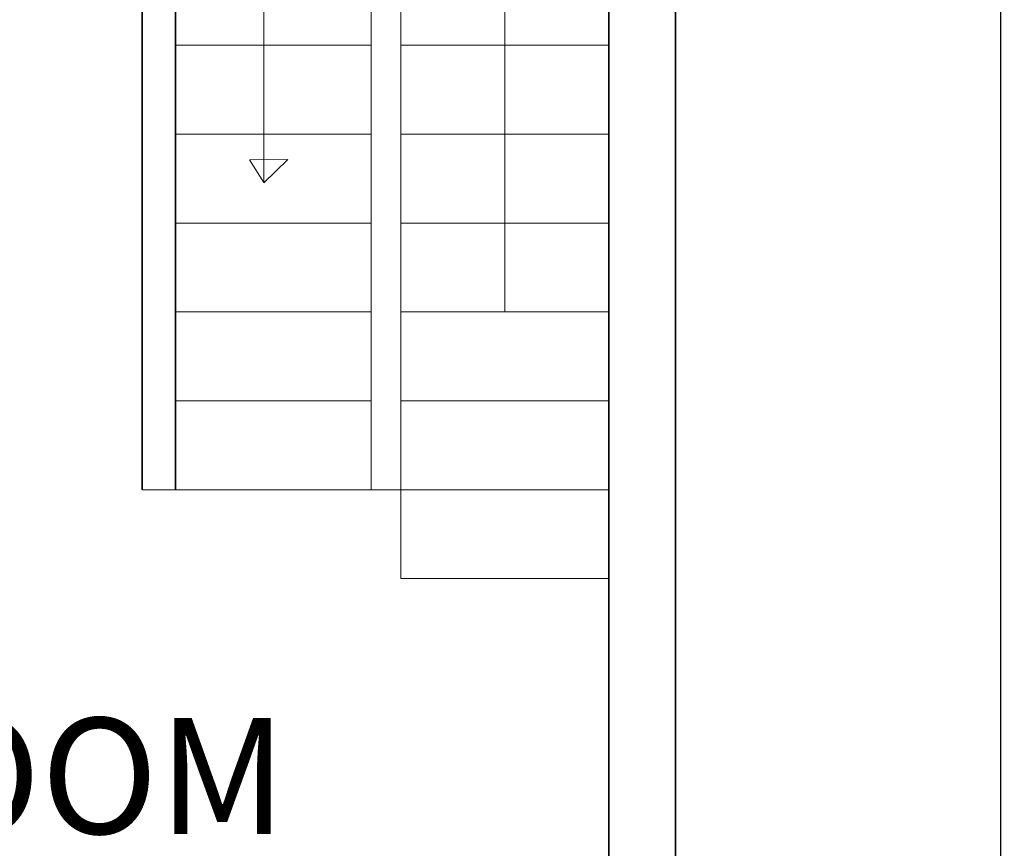
# Model space of a CAD drawing. Units: inches. Extents: x -26 to 788, y -42 to 505.
# Tile 6 of 9: x 219 to 352, y 262 to 374. Entities that reach past the tile are written whole.
import ezdxf

# ---------------------------------------------------------------- set-up
doc = ezdxf.new("R2010")
doc.units = ezdxf.units.IN
doc.header["$MEASUREMENT"] = 0
for name, color, linetype, lineweight in [('A-ANNO-DIMS', 2, 'Continuous', 18), ('A-AREA-IDEN', 7, 'Continuous', 18), ('A-FLOR-STRS', 7, 'Continuous', 18), ('A-WALL', 7, 'Continuous', 35)]:
    doc.layers.add(name, color=color, linetype=linetype, lineweight=lineweight)
doc.styles.get("Standard").update_dxf_attribs({"font": 'arial.ttf'})
doc.dimstyles.get("Standard").update_dxf_attribs({"dimtxt": 0.18, "dimasz": 0.18, "dimexe": 0.18, "dimexo": 0.0625, "dimgap": 0.09, "dimtad": 0, "dimtih": 1, "dimtoh": 1, "dimdec": 4, "dimzin": 0, "dimdsep": 46, "dimtxsty": 'Standard', "dimcen": 0.09, "dimadec": 0, "dimazin": 0, "dimtfac": 1, "dimtdec": 4, "dimtofl": 0, "dimtmove": 0, "dimatfit": 3, "dimfxl": 1, "dimtolj": 1, "dimtzin": 0, "dimarcsym": 0})

# ---------------------------------------------------------------- blocks, each defined once
blk = doc.blocks.new('*D8')
at = {"layer": 'A-ANNO-DIMS', "color": 0, "lineweight": -2, "transparency": 16777216}
for p, q in [((307.52, 431.12), (351.51, 431.12)), ((351.33, 430.94), (351.33, 216.8)), ((351.33, 2.3), (351.33, 216.44)), ((307.52, 2.12), (351.51, 2.12))]:
    blk.add_line(p, q, dxfattribs=at)
at = {"layer": 'A-ANNO-DIMS', "color": 0, "transparency": 16777216}
for points in [[(351.3, 430.94), (351.36, 430.94), (351.33, 431.12)], [(351.3, 2.3), (351.36, 2.3), (351.33, 2.12)]]:
    blk.add_solid(points, dxfattribs=at)
at = {"layer": 'Defpoints', "color": 0, "transparency": 16777216}
for p in [(307.45, 431.12), (307.45, 2.12), (351.33, 2.12)]:
    blk.add_point(p, dxfattribs=at)
at = {"layer": 'A-ANNO-DIMS', "color": 0, "transparency": 16777216, "insert": (351.33, 216.62), "char_height": 0.18, "attachment_point": 5}
blk.add_mtext('\\A1;429.0000', dxfattribs=at)
blk = doc.blocks.new('STAIR-RETURN')
for p, q in [((30.9, 12), (30.9, 123.91)), ((34.9, 0), (34.9, 123.91)), ((4.5, 96), (30.9, 96)), ((34.9, 96), (63, 96)), ((4.5, 84), (30.9, 84)), ((34.9, 84), (63, 84)), ((4.5, 72), (30.9, 72)), ((34.9, 72), (63, 72)), ((4.5, 60), (30.9, 60)), ((34.9, 60), (63, 60)), ((4.5, 48), (30.9, 48)), ((34.9, 48), (63, 48)), ((4.5, 36), (30.9, 36)), ((34.9, 36), (63, 36)), ((4.5, 24), (30.9, 24)), ((34.9, 24), (63, 24)), ((0, 12), (63, 12)), ((34.9, 0), (63, 0))]:
    blk.add_line(p, q)
blk.add_lwpolyline([(48.95, 36), (48.95, 108.21), (16.43, 108.21), (16.43, 53.45), (19.67, 56.58), (14.49, 56.53), (16.4, 53.46)])

msp = doc.modelspace()

# ---------------------------------------------------------------- linework, layer by layer
at = {"layer": 'A-WALL'}
for p, q in [((307.45497, 308.37421), (307.45497, 431.11777)), ((235.45497, 310.20306), (235.45497, 422.11777)), ((239.95497, 310.20306), (239.95497, 422.11777)), ((298.45497, 164.11777), (298.45497, 422.11777)), ((307.45497, 2.11777), (307.45497, 308.37421))]:
    msp.add_line(p, q, dxfattribs=at)

# ---------------------------------------------------------------- block references
at = {"layer": 'A-FLOR-STRS'}
msp.add_blockref('STAIR-RETURN', (235.455, 298.203), dxfattribs=at)

# ---------------------------------------------------------------- texts
at = {"layer": 'A-AREA-IDEN'}
msp.add_text('LIVING ROOM', height=15.6450193, dxfattribs=at).set_placement((121.09986, 263.74771))

# ---------------------------------------------------------------- dimensions: what is measured, and where the dimension line sits
at = {"layer": 'A-ANNO-DIMS'}
dim = msp.add_linear_dim(base=(351.33135, 2.11777), p1=(307.45497, 431.11777), p2=(307.45497, 2.11777), angle=90, dimstyle='Standard', override={"dimclrd": 0, "dimclre": 0, "dimclrt": 0}, dxfattribs=at)
dim.commit()
dim.dimension.update_dxf_attribs({"geometry": '*D8', "text_midpoint": (351.33135, 216.61777)})

doc.saveas('drawing.dxf')
